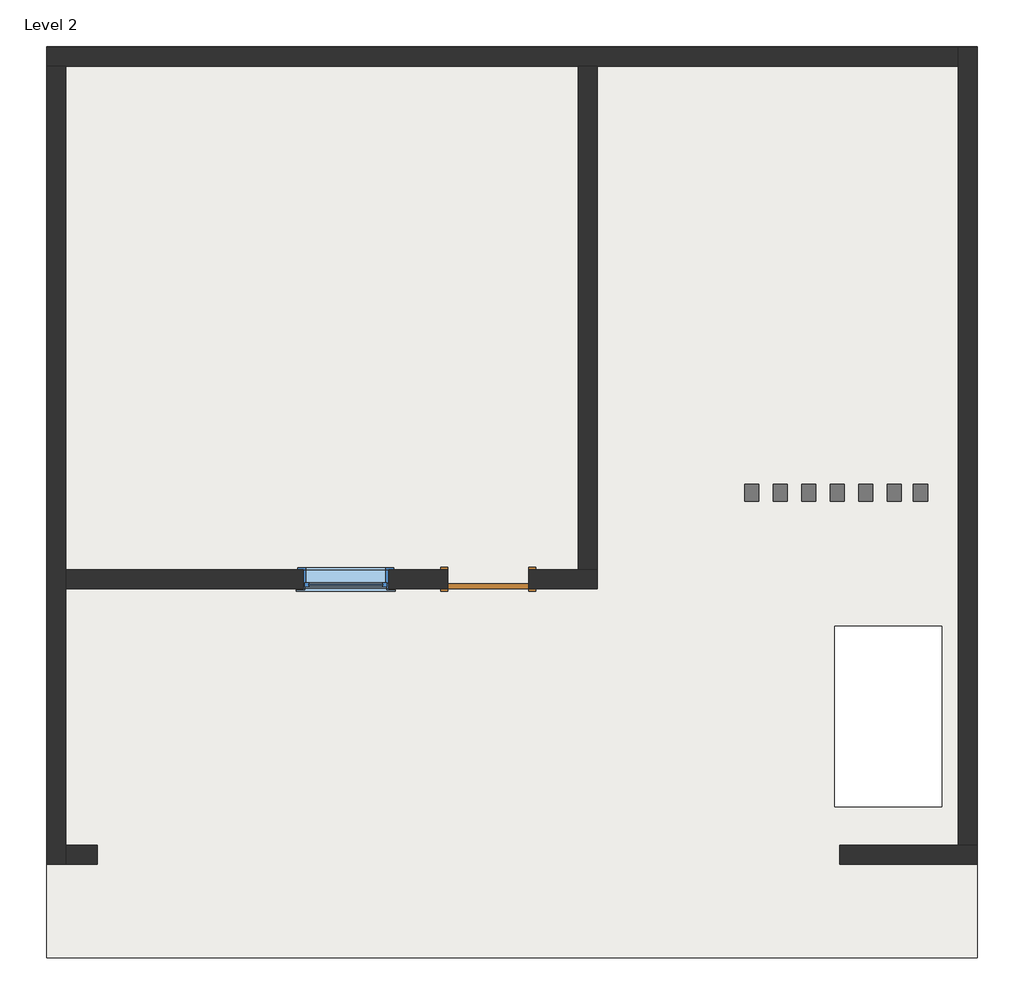
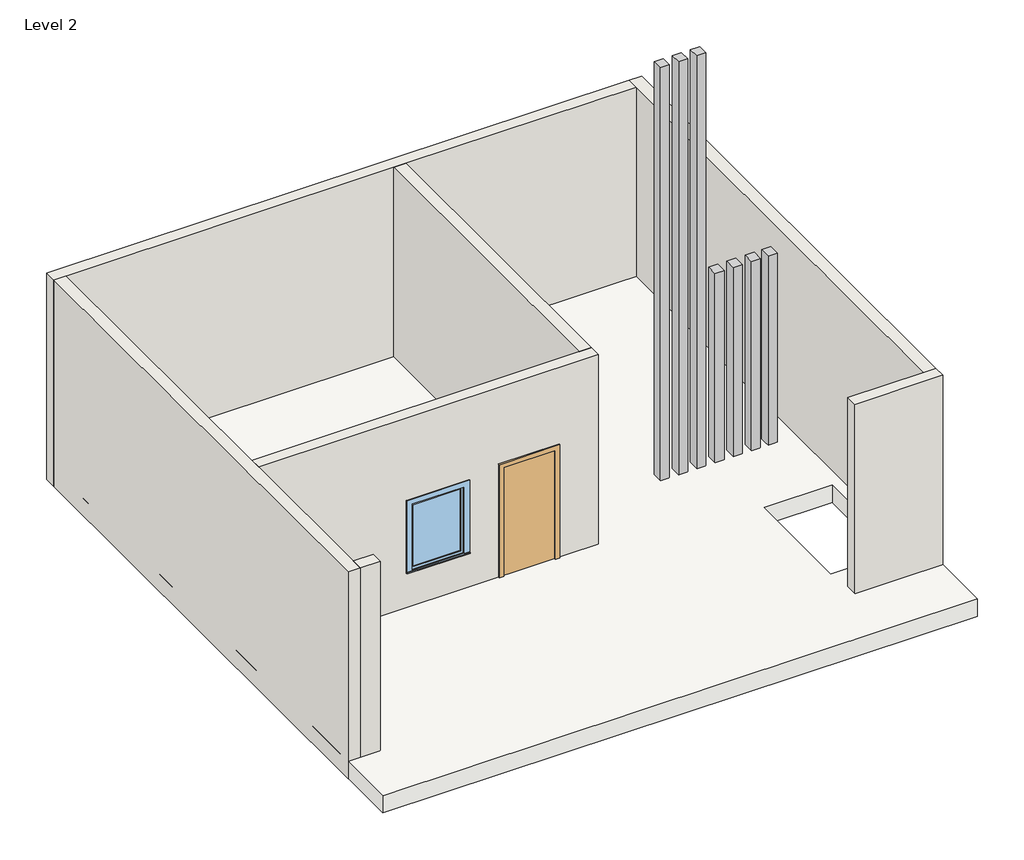
# One storey: 7 proxies, 6 walls, 1 door, 1 roof, 1 window.
"""IFC4 building model written with IfcOpenShell, lengths in millimetres."""

from ifc_helpers import new_model, si_unit, frame, origin, place, context, project, spatial, polyline, outline, extrude, faceted_brep, transform, mapped, element, save
from components import door_10fd3a06, window_bec2521a

model = new_model("IFC4")

# Units and contexts
model_context = context("Model", 3, world=origin())
ifc_project = project(units=[si_unit("LENGTHUNIT", "METRE", prefix="MILLI")], contexts=[model_context])

# Site, building, storey
site = spatial("IfcSite", under=ifc_project)
building = spatial("IfcBuilding", under=site)
storey = spatial("IfcBuildingStorey", under=building, Name="Level 2", Elevation=3657.6)

# Proxies
placement = place(None, origin())
element("IfcBuildingElementProxy", 1, Name="Reveal", ObjectType="Reveal", at=placement, inside=storey, context=model_context, shape_type="SweptSolid", body=[
    extrude(outline(polyline([(-5345.5931367, 6437.3997066), (-5345.5931367, 6620.2797066), (-5193.1931367, 6620.2797066), (-5193.1931367, 6437.3997066), (-5345.5931367, 6437.3997066)])), frame((0.0, 0.0, 3962.4), z_axis=(0.0, 0.0, 1.0), x_axis=(1.0, 0.0, 0.0)), (0.0, 0.0, 1.0), 7315.2),
])
element("IfcBuildingElementProxy", 2, Name="Reveal", ObjectType="Reveal", at=placement, inside=storey, context=model_context, shape_type="SweptSolid", body=[
    extrude(outline(polyline([(-5040.7931367, 6437.3997066), (-5040.7931367, 6620.2797066), (-4888.3931367, 6620.2797066), (-4888.3931367, 6437.3997066), (-5040.7931367, 6437.3997066)])), frame((0.0, 0.0, 3962.4), z_axis=(0.0, 0.0, 1.0), x_axis=(1.0, 0.0, 0.0)), (0.0, 0.0, 1.0), 7315.2),
])
element("IfcBuildingElementProxy", 3, Name="Reveal", ObjectType="Reveal", at=placement, inside=storey, context=model_context, shape_type="SweptSolid", body=[
    extrude(outline(polyline([(-4735.9931367, 6437.3997066), (-4735.9931367, 6620.2797066), (-4583.5931367, 6620.2797066), (-4583.5931367, 6437.3997066), (-4735.9931367, 6437.3997066)])), frame((0.0, 0.0, 3962.4), z_axis=(0.0, 0.0, 1.0), x_axis=(1.0, 0.0, 0.0)), (0.0, 0.0, 1.0), 7315.2),
])
element("IfcBuildingElementProxy", 4, Name="Reveal", ObjectType="Reveal", at=placement, inside=storey, context=model_context, shape_type="SweptSolid", body=[
    extrude(outline(polyline([(-4431.1931367, 6437.3997066), (-4431.1931367, 6620.2797066), (-4278.7931367, 6620.2797066), (-4278.7931367, 6437.3997066), (-4431.1931367, 6437.3997066)])), frame((0.0, 0.0, 3962.4), z_axis=(0.0, 0.0, 1.0), x_axis=(1.0, 0.0, 0.0)), (0.0, 0.0, 1.0), 3352.8),
])
element("IfcBuildingElementProxy", 5, Name="Reveal", ObjectType="Reveal", at=placement, inside=storey, context=model_context, shape_type="SweptSolid", body=[
    extrude(outline(polyline([(-4126.3931367, 6437.3997066), (-4126.3931367, 6620.2797066), (-3973.9931367, 6620.2797066), (-3973.9931367, 6437.3997066), (-4126.3931367, 6437.3997066)])), frame((0.0, 0.0, 3962.4), z_axis=(0.0, 0.0, 1.0), x_axis=(1.0, 0.0, 0.0)), (0.0, 0.0, 1.0), 3352.8),
])
element("IfcBuildingElementProxy", 6, Name="Reveal", ObjectType="Reveal", at=placement, inside=storey, context=model_context, shape_type="SweptSolid", body=[
    extrude(outline(polyline([(-3821.5931367, 6437.3997066), (-3821.5931367, 6620.2797066), (-3669.1931367, 6620.2797066), (-3669.1931367, 6437.3997066), (-3821.5931367, 6437.3997066)])), frame((0.0, 0.0, 3962.4), z_axis=(0.0, 0.0, 1.0), x_axis=(1.0, 0.0, 0.0)), (0.0, 0.0, 1.0), 3352.8),
])
element("IfcBuildingElementProxy", 7, Name="Reveal", ObjectType="Reveal", at=placement, inside=storey, context=model_context, shape_type="SweptSolid", body=[
    extrude(outline(polyline([(-3542.1931367, 6437.3997066), (-3542.1931367, 6620.2797066), (-3389.7931367, 6620.2797066), (-3389.7931367, 6437.3997066), (-3542.1931367, 6437.3997066)])), frame((0.0, 0.0, 3962.4), z_axis=(0.0, 0.0, 1.0), x_axis=(1.0, 0.0, 0.0)), (0.0, 0.0, 1.0), 3352.8),
])

# Door
door_shape = door_10fd3a06(model_context)
element("IfcDoor", 8, ObjectType="Door-Single-Panel : 34\" x 80\"", at=placement, inside=storey, context=model_context, shape_type="MappedRepresentation", body=[
    mapped(door_shape, transform((-8088.7931367, 5604.2797066, 3860.8), x_axis=(-1.0, 0.0, 0.0), y_axis=(0.0, -1.0, 0.0), z_axis=(0.0, 0.0, 1.0))),
])

# Roof
element("IfcRoof", 9, ObjectType="Generic - 12\"", at=placement, inside=storey, context=model_context, shape_type="SweptSolid", body=[
    extrude(outline(polyline([(-12813.1931367, 11300.8300502), (-2856.3931367, 11300.8300502), (-2856.3931367, 1552.6285778), (-12813.1931367, 1552.6285778), (-12813.1931367, 11300.8300502)]), holes=[polyline([(-3237.3931367, 3169.7811291), (-3237.3931367, 5100.1811291), (-4380.3931367, 5100.1811291), (-4380.3931367, 3169.7811291), (-3237.3931367, 3169.7811291)])]), frame((0.0, 0.0, 3657.6), z_axis=(0.0, 0.0, 1.0), x_axis=(1.0, 0.0, 0.0)), (0.0, 0.0, 1.0), 304.8),
])

# Walls
element("IfcWall", 10, ObjectType="Generic - 8\"", at=placement, inside=storey, context=model_context, shape_type="Brep", body=[
    faceted_brep([(-12813.1931367, 11090.6797066, 3657.6), (-12609.9931367, 11090.6797066, 3657.6), (-7123.5931367, 11090.6797066, 3657.6), (-6920.3931367, 11090.6797066, 3657.6), (-3059.5931367, 11090.6797066, 3657.6), (-3059.5931367, 11090.6797066, 7315.2), (-6920.3931367, 11090.6797066, 7315.2), (-7123.5931367, 11090.6797066, 7315.2), (-12609.9931367, 11090.6797066, 7315.2), (-12813.1931367, 11090.6797066, 7315.2), (-12813.1931367, 11293.8797066, 3657.6), (-12813.1931367, 11293.8797066, 7315.2), (-3059.5931367, 11293.8797066, 7315.2), (-3059.5931367, 11293.8797066, 3657.6)], [[[0, 1, 2, 3, 4, 5, 6, 7, 8, 9]], [[10, 11, 12, 13]], [[4, 3, 2, 1, 0, 10, 13]], [[9, 8, 7, 6, 5, 12, 11]], [[0, 9, 11, 10]], [[5, 4, 13, 12]]]),
])
element("IfcWall", 11, ObjectType="Generic - 8\"", at=placement, inside=storey, context=model_context, shape_type="Brep", body=[
    faceted_brep([(-12609.9931367, 2556.2797066, 3657.6), (-12609.9931367, 2759.4797066, 3657.6), (-12609.9931367, 5502.6797066, 3657.6), (-12609.9931367, 5705.8797066, 3657.6), (-12609.9931367, 11090.6797066, 3657.6), (-12609.9931367, 11090.6797066, 7315.2), (-12609.9931367, 5705.8797066, 7315.2), (-12609.9931367, 5502.6797066, 7315.2), (-12609.9931367, 2759.4797066, 7315.2), (-12609.9931367, 2556.2797066, 7315.2), (-12813.1931367, 2556.2797066, 3657.6), (-12813.1931367, 2556.2797066, 7315.2), (-12813.1931367, 11090.6797066, 7315.2), (-12813.1931367, 11090.6797066, 3657.6)], [[[0, 1, 2, 3, 4, 5, 6, 7, 8, 9]], [[10, 11, 12, 13]], [[4, 3, 2, 1, 0, 10, 13]], [[9, 8, 7, 6, 5, 12, 11]], [[0, 9, 11, 10]], [[5, 4, 13, 12]]]),
])
element("IfcWall", 12, ObjectType="Generic - 8\"", at=placement, inside=storey, context=model_context, shape_type="Brep", body=[
    faceted_brep([(-12609.9931367, 2759.4797066, 7315.2), (-12271.0796378, 2759.4797066, 7315.2), (-12271.0796378, 2759.4797066, 3657.6), (-12609.9931367, 2759.4797066, 3657.6), (-12609.9931367, 2556.2797066, 7315.2), (-12609.9931367, 2556.2797066, 3657.6), (-12271.0796378, 2556.2797066, 3657.6), (-12271.0796378, 2556.2797066, 7315.2)], [[[0, 1, 2, 3]], [[4, 5, 6, 7]], [[0, 3, 5, 4]], [[1, 0, 4, 7]], [[2, 1, 7, 6]], [[3, 2, 6, 5]]]),
    faceted_brep([(-2856.3931367, 2759.4797066, 3657.6), (-3059.5931367, 2759.4797066, 3657.6), (-4329.8030581, 2759.4797066, 3657.6), (-4329.8030581, 2759.4797066, 7315.2), (-3059.5931367, 2759.4797066, 7315.2), (-2856.3931367, 2759.4797066, 7315.2), (-2856.3931367, 2556.2797066, 3657.6), (-2856.3931367, 2556.2797066, 7315.2), (-4329.8030581, 2556.2797066, 7315.2), (-4329.8030581, 2556.2797066, 3657.6)], [[[0, 1, 2, 3, 4, 5]], [[6, 7, 8, 9]], [[0, 5, 7, 6]], [[2, 1, 0, 6, 9]], [[3, 2, 9, 8]], [[5, 4, 3, 8, 7]]]),
])
element("IfcWall", 13, ObjectType="Generic - 8\"", at=placement, inside=storey, context=model_context, shape_type="Brep", body=[
    faceted_brep([(-3059.5931367, 11293.8797066, 3657.6), (-3059.5931367, 11090.6797066, 3657.6), (-3059.5931367, 2759.4797066, 3657.6), (-3059.5931367, 2759.4797066, 7315.2), (-3059.5931367, 11090.6797066, 7315.2), (-3059.5931367, 11293.8797066, 7315.2), (-2856.3931367, 11293.8797066, 3657.6), (-2856.3931367, 11293.8797066, 7315.2), (-2856.3931367, 2759.4797066, 7315.2), (-2856.3931367, 2759.4797066, 3657.6)], [[[0, 1, 2, 3, 4, 5]], [[6, 7, 8, 9]], [[2, 1, 0, 6, 9]], [[5, 4, 3, 8, 7]], [[0, 5, 7, 6]], [[3, 2, 9, 8]]]),
])
element("IfcWall", 14, ObjectType="Generic - 8\"", at=placement, inside=storey, context=model_context, shape_type="Brep", body=[
    faceted_brep([(-12609.9931367, 5502.6797066, 3657.6), (-6920.3931367, 5502.6797066, 3657.6), (-6920.3931367, 5502.6797066, 7315.2), (-12609.9931367, 5502.6797066, 7315.2), (-7656.9931367, 5502.6797066, 3860.8), (-8520.5931367, 5502.6797066, 3860.8), (-8520.5931367, 5502.6797066, 5892.8), (-7656.9931367, 5502.6797066, 5892.8), (-10069.9931367, 5502.6797066, 5791.2), (-9155.5931367, 5502.6797066, 5791.2), (-9155.5931367, 5502.6797066, 4572.0), (-10069.9931367, 5502.6797066, 4572.0), (-12609.9931367, 5705.8797066, 3657.6), (-12609.9931367, 5705.8797066, 7315.2), (-7123.5931367, 5705.8797066, 7315.2), (-6920.3931367, 5705.8797066, 7315.2), (-6920.3931367, 5705.8797066, 3657.6), (-7123.5931367, 5705.8797066, 3657.6), (-7656.9931367, 5705.8797066, 3860.8), (-7656.9931367, 5705.8797066, 5892.8), (-8520.5931367, 5705.8797066, 5892.8), (-8520.5931367, 5705.8797066, 3860.8), (-10069.9931367, 5705.8797066, 5791.2), (-10069.9931367, 5705.8797066, 4572.0), (-9155.5931367, 5705.8797066, 4572.0), (-9155.5931367, 5705.8797066, 5791.2)], [[[0, 1, 2, 3], [4, 5, 6, 7], [8, 9, 10, 11]], [[12, 13, 14, 15, 16, 17], [18, 19, 20, 21], [22, 23, 24, 25]], [[1, 0, 12, 17, 16]], [[3, 2, 15, 14, 13]], [[0, 3, 13, 12]], [[2, 1, 16, 15]], [[5, 4, 18, 21]], [[6, 5, 21, 20]], [[7, 6, 20, 19]], [[4, 7, 19, 18]], [[23, 22, 8, 11]], [[24, 23, 11, 10]], [[25, 24, 10, 9]], [[22, 25, 9, 8]]]),
])
element("IfcWall", 15, ObjectType="Generic - 8\"", at=placement, inside=storey, context=model_context, shape_type="SweptSolid", body=[
    extrude(outline(polyline([(-6920.3931367, 11090.6797066), (-6920.3931367, 5705.8797066), (-7123.5931367, 5705.8797066), (-7123.5931367, 11090.6797066), (-6920.3931367, 11090.6797066)])), frame((0.0, 0.0, 3657.6), z_axis=(0.0, 0.0, 1.0), x_axis=(1.0, 0.0, 0.0)), (0.0, 0.0, 1.0), 3657.6),
])

# Window
window_shape = window_bec2521a(model_context)
element("IfcWindow", 16, ObjectType="Fixed with Trim : 36\" x 48\"", at=placement, inside=storey, context=model_context, shape_type="MappedRepresentation", body=[
    mapped(window_shape, transform((-9650.8931367, 5604.2797066, 3657.6), x_axis=(-1.0, 0.0, 0.0), y_axis=(0.0, -1.0, 0.0), z_axis=(0.0, 0.0, 1.0))),
])

save(model, "model.ifc")

# Revit data of these elements
# Type "Door-Single-Panel : 34\" x 80\""
#   Type Mark = "8"
#   Construction Type Id = "DOOR"
#   Assembly Code = "C1020300"
#   Analytic Construction = "Wooden"
#   Thickness = 0' - 2"
#   Thermal Resistance (R) = 2.5876 (h·ft²·°F)/BTU
#   Swing Angle [instance default] = 90.00°
#   Heat Transfer Coefficient (U) = 0.3865 BTU/(h·ft²·°F)
#   Height = 6' - 8"
#   Trim Projection Ext = 0' - 1"
#   Trim Projection Int = 0' - 1"
#   Trim Width = 0' - 3"
#   Width = 2' - 10"
#   Define Thermal Properties by = 1
#   Panel Material = Wood - Birch - Solid Stained Light Low Gloss
#   Trim Material = Paint - Sienna
#   Visual Light Transmittance = 0
#   Solar Heat Gain Coefficient = 0
#   Function = (empty or 0)
#   Wall Closure = (empty or 0)
# Type "Generic - 12\""
#   Assembly Code = "B1020"
#   Layers, outside or top first: 1' - 0" no material (function 1)
# Type "Generic - 8\""
#   Assembly Code = "B2010"
#   Layers, outside or top first: 0' - 8" no material (function 1)
# Type "Fixed with Trim : 36\" x 48\""
#   Type Mark = "13"
#   Construction Type Id = "GSP4R"
#   Assembly Code = "B2020100"
#   Analytic Construction = "1/8 in Pilkington single glazing"
#   Visual Light Transmittance = 0.9
#   Solar Heat Gain Coefficient = 0.78
#   Heat Transfer Coefficient (U) = 0.6496 BTU/(h·ft²·°F)
#   Height = 4' - 0"
#   Default Sill Height = 3' - 0"
#   Trim Projection - Ext. = 0' - 0 1/2"
#   Trim Projection - Int. = 0' - 0 3/4"
#   Trim Width - Exterior = 0' - 3 1/2"
#   Trim Width - Interior = 0' - 3 1/2"
#   Width = 3' - 0"
#   Window Inset = 0' - 0 3/4"
#   Define Thermal Properties by = 1
#   Glass Pane Material = Glass
#   Sash Material = Sash
#   Trim Exterior Material = Trim
#   Trim Interior Material = Trim
#   Wall Closure = (empty or 0)
# Element 8 (IfcDoor, "Door-Single-Panel : 34\" x 80\"")
#   Swing Angle = 90.00°
#   Phase Created = New Construction
#   Materials on its faces: "Paint - Sienna", "Wood - Birch - Solid Stained Light Low Gloss"
# Element 9 (IfcRoof, "Generic - 12\"")
#   built-in parameter 1001705 = 13 (stored number, unit not read)
#   built-in parameter 1001710 = 33615
#   Phase Created = New Construction
#   Materials on its faces: "Default Roof"
# Elements 10, 11, 12, 13, 14, 15 (IfcWall, "Generic - 8\"")
#   Top Offset = 0' - 0"
#   Base Offset = 0' - 0"
#   Unconnected Height = 12' - 0"
#   wall height = 12' - 0"
#   Phase Created = New Construction
#   Base Constraint = Level 2
#   Materials on its faces: "Default Wall"
# Element 16 (IfcWindow, "Fixed with Trim : 36\" x 48\"")
#   Mark = "2"
#   Phase Created = New Construction
#   Materials on its faces: "Sash", "Trim", "Glass"
# Materials
#   "Wood - Birch - Solid Stained Light Low Gloss": class "Wood", colour RGB 210 159 95, transparency 0, Cost = 0
#   "Paint - Sienna": colour RGB 118 70 51, transparency 0, Cost = 0
#   "Glass": class "Glass", colour RGB 0 128 192, transparency 0.75, Description = "Soda Lime Glass", Cost = 0
#   "Sash": class "Wood", colour RGB 224 178 126, transparency 0
#   "Trim": class "Wood", colour RGB 224 178 126, transparency 0
#   "Default Roof": colour RGB 88 101 114, transparency 0
#   "Default Wall": colour RGB 128 128 128, transparency 0
